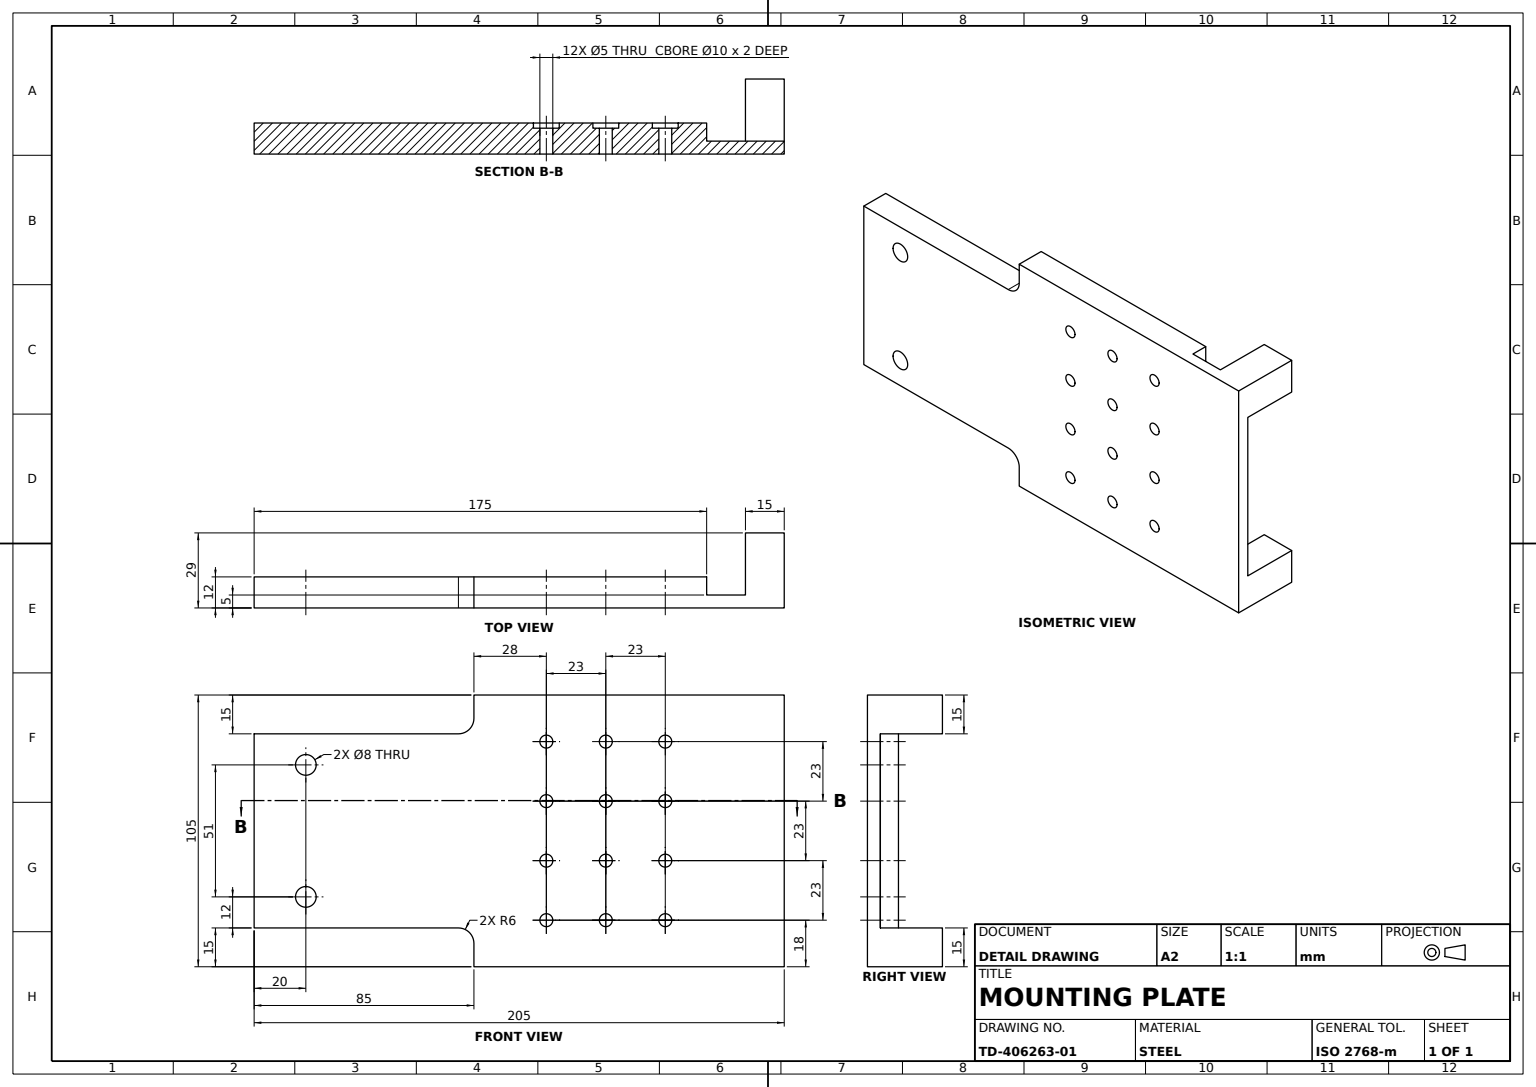
SolidWorks part; units mm, degrees
material "Plain Carbon Steel"
ref_plane "Front Plane" through (0, 0, 0) normal (0, 0, 1) x (1, 0, 0)
ref_plane "Top Plane" through (0, 0, 0) normal (0, 1, 0) x (1, 0, 0)
ref_plane "Right Plane" through (0, 0, 0) normal (1, 0, 0) x (0, 0, -1)
sketch "Base Plate Sketch" plane through (0, 0, 0) normal (0, 0, 1) x (1, 0, 0)
  line L0 (0, 0) -> (85, 0)
  line L1 (85, 0) -> (85, 75)
  line L2 (85, 75) -> (0, 75)
  line L3 (0, 75) -> (0, 0)
  dimension "D1" = 85
  dimension "D2" = 75
extrude "Base Plate 85x75" add sketch "Base Plate Sketch" along normal blind 12
sketch "Plate Extension Sketch" plane through (0, 0, 12) normal (0, 0, 1) x (1, 0, 0)
  line L0 (0, 37.5) -> (175, 37.5)
  line L1 (0, 75) -> (0, 0) construction
  line L2 (175, -15) -> (175, 90)
  line L3 (175, 90) -> (85, 90)
  line L4 (85, 90) -> (85, 75)
  line L5 (175, -15) -> (85, -15)
  line L6 (85, -15) -> (85, 0)
  line L7 (85, 75) -> (85, 0)
  point P7 (175, 37.5)
  line M3 (85, 0) -> (85, 75)
  dimension "D1" = 175
  dimension "D2" = 52.5
extrude "Plate Extension" add sketch "Plate Extension Sketch" against normal blind 12 contours L3 L4 L0 L2 M3 | L6 L5 L2 L0 M3
fillet "Notch Fillet R6 A" radius 6 1 edges at (85, 75, 6)
fillet "Notch Fillet R6 B" radius 6 1 edges at (85, 0, 6)
sketch "End Flange Sketch" plane through (0, 0, 12) normal (0, 0, 1) x (1, 0, 0)
  line L0 (175, 90) -> (205, 90)
  line L1 (205, 90) -> (205, -15)
  line L2 (205, -15) -> (175, -15)
  line L3 (175, -15) -> (175, 90)
  dimension "D1" = 30
extrude "End Flange" add sketch "End Flange Sketch" against normal blind 5
sketch "Side Tab 1 Sketch" plane through (0, 90, 0) normal (0, 1, 0) x (1, 0, 0)
  line L0 (205, -7) -> (190, -7)
  line L2 (205, -7) -> (175, -7) construction
  line L3 (190, -7) -> (190, 17)
  line L4 (190, 17) -> (205, 17)
  line L5 (205, 17) -> (205, -7)
  dimension "D1" = 15
  dimension "D2" = 24
extrude "Side Tab 1" add sketch "Side Tab 1 Sketch" against normal blind 15
sketch "Side Tab 2 Sketch" plane through (0, -15, 0) normal (0, -1, 0) x (1, 0, 0)
  line L0 (190, 7) -> (190, -17)
  line L1 (190, -17) -> (205, -17)
  line L2 (205, -17) -> (205, 7)
  line L3 (205, 7) -> (190, 7)
extrude "Side Tab 2" add sketch "Side Tab 2 Sketch" against normal blind 15
sketch "Counterbore Grid Sketch" plane through (0, 0, 0) normal (0, 0, -1) x (-1, 0, 0)
  line L0 (-175, 90) -> (-85, 90) construction
  line L1 (-85, 90) -> (-85, 81) construction
  line L2 (-85, -6) -> (-85, -15) construction
  line L3 (-205, 37.5) -> (0, 37.5)
  line L5 (-205, 0) -> (-205, 75) construction
  line L6 (0, 75) -> (0, 0) construction
  circle A0 centre (-159, 72) radius 5
  circle A1 centre (-136, 72) radius 5
  circle A2 centre (-113, 72) radius 5
  circle A3 centre (-113, 49) radius 5
  circle A4 centre (-113, 26) radius 5
  circle A5 centre (-113, 3) radius 5
  circle A6 centre (-136, 3) radius 5
  circle A7 centre (-159, 3) radius 5
  circle A8 centre (-159, 49) radius 5
  circle A9 centre (-159, 26) radius 5
  circle A10 centre (-136, 26) radius 5
  circle A11 centre (-136, 49) radius 5
  dimension "D1" = 10
  dimension "D2" = 10
  dimension "D3" = 10
  dimension "D4" = 10
  dimension "D5" = 10
  dimension "D6" = 10
  dimension "D7" = 10
  dimension "D8" = 10
  dimension "D9" = 10
  dimension "D10" = 10
  dimension "D11" = 10
  dimension "D12" = 10
  dimension "D13" = 28
  dimension "D14" = 28
  dimension "D15" = 18
  dimension "D16" = 23
  dimension "D17" = 18
  dimension "D18" = 23
  dimension "D19" = 23
  dimension "D20" = 11.5
  dimension "D21" = 28
  dimension "D22" = 11.5
  dimension "D23" = 28
  dimension "D24" = 23
  dimension "D25" = 23
  dimension "D26" = 23
  dimension "D27" = 11.5
  dimension "D28" = 23
  dimension "D29" = 23
  dimension "D30" = 23
  dimension "D31" = 23
  dimension "D32" = 23
  dimension "D33" = 23
  dimension "D34" = 23
  dimension "D35" = 23
  dimension "D36" = 23
extrude "Counterbores 12xØ10" cut sketch "Counterbore Grid Sketch" against normal blind 2 contours A0 | A1 | A2 | A3 | A11 | A8 | A9 | A10 | A4 | A5 | A6 | A7
sketch "Hole Grid Sketch" plane through (0, 0, 2) normal (0, 0, -1) x (-1, 0, 0)
  circle A0 centre (-159, 72) radius 2.5
  circle A1 centre (-136, 72) radius 2.5
  circle A2 centre (-113, 72) radius 2.5
  circle A3 centre (-113, 49) radius 2.5
  circle A4 centre (-136, 49) radius 2.5
  circle A5 centre (-159, 49) radius 2.5
  circle A6 centre (-159, 26) radius 2.5
  circle A7 centre (-136, 26) radius 2.5
  circle A8 centre (-113, 26) radius 2.5
  circle A9 centre (-159, 3) radius 2.5
  circle A10 centre (-136, 3) radius 2.5
  circle A11 centre (-113, 3) radius 2.5
  dimension "D1" = 5
  dimension "D2" = 5
  dimension "D3" = 5
  dimension "D4" = 5
  dimension "D5" = 5
  dimension "D6" = 5
  dimension "D7" = 5
  dimension "D8" = 5
  dimension "D9" = 5
  dimension "D10" = 5
  dimension "D11" = 5
  dimension "D12" = 5
extrude "Hole Grid 12xØ5" cut sketch "Hole Grid Sketch" against normal blind 10
sketch "Mounting Holes Sketch" plane through (0, 0, 0) normal (0, 0, -1) x (-1, 0, 0)
  line L0 (0, 75) -> (0, 0) construction
  line L1 (-79, 75) -> (0, 75) construction
  line L2 (0, 0) -> (-79, 0) construction
  circle A0 centre (-20, 63) radius 4
  circle A1 centre (-20, 12) radius 4
  dimension "D1" = 8
  dimension "D2" = 8
  dimension "D3" = 20
  dimension "D4" = 12
  dimension "D5" = 20
  dimension "D6" = 12
extrude "Mounting Holes 2xØ8" cut sketch "Mounting Holes Sketch" against normal blind 15
